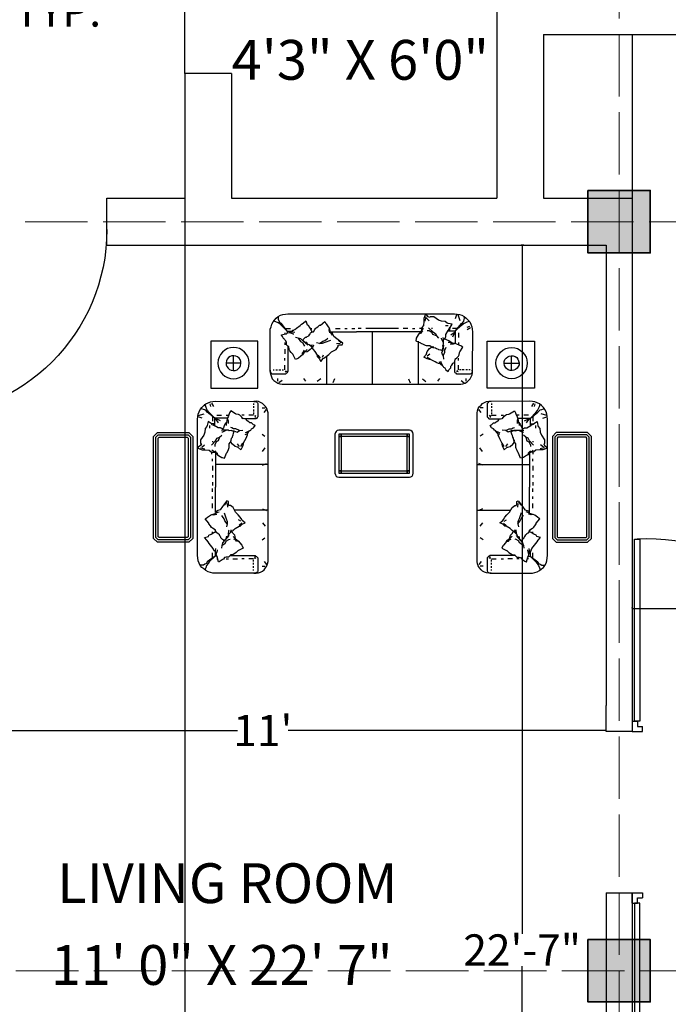
# Model space of a CAD drawing. Units: inches. Extents: x -113 to 5399, y -1393 to 3302.
# Tile 4 of 40: x 1068 to 1193, y 271 to 460. Entities that reach past the tile are written whole.
import ezdxf

# ---------------------------------------------------------------- set-up
doc = ezdxf.new("R2010")
doc.units = ezdxf.units.IN
doc.header["$MEASUREMENT"] = 0
doc.linetypes.add('ACAD_ISO02W100', pattern=[15, 12, -3])
doc.layers.add('24', color=7, linetype='Continuous')
for name, color, linetype, lineweight in [('A-ANNO-DIMS', 254, 'Continuous', 18), ('A-AREA-IDEN', 4, 'Continuous', 18), ('A-COLS', 7, 'Continuous', 35), ('doors', 2, 'Continuous', 25), ('furniture', 131, 'Continuous', 18), ('GRIDS', 7, 'ACAD_ISO02W100', 13), ('walls', 1, 'Continuous', 25)]:
    doc.layers.add(name, color=color, linetype=linetype, lineweight=lineweight)
doc.styles.get("Standard").update_dxf_attribs({"font": 'arial.ttf'})
doc.dimstyles.get("Standard").update_dxf_attribs({"dimtxt": 6, "dimasz": 0.18, "dimexe": 0.18, "dimexo": 0.0625, "dimgap": 0.09, "dimtad": 0, "dimtih": 1, "dimtoh": 1, "dimdec": 1, "dimzin": 0, "dimdsep": 46, "dimlunit": 4, "dimtxsty": 'Standard', "dimblk": 'ARCHTICK', "dimcen": 0.09, "dimadec": 0, "dimazin": 0, "dimtfac": 1, "dimtdec": 1, "dimtofl": 0, "dimtmove": 0, "dimatfit": 3, "dimfxl": 1, "dimtolj": 1, "dimtzin": 0, "dimarcsym": 0})

# ---------------------------------------------------------------- blocks, each defined once
blk = doc.blocks.new('*U3')
for p, q in [((0, 0), (0, -6)), ((36, 0), (36, -6))]:
    blk.add_line(p, q)
blk.add_lwpolyline([(0, 0), (0, 36), (1.75, 36), (1.75, 0)], close=True)
blk.add_arc((0, 0), 36, 0, 90)
blk = doc.blocks.new('DL13712')
at = {"layer": '24'}
for p, q in [((33, 28.5), (-34, 28.5)), ((33.5, -29.5), (-10, -29.5))]:
    blk.add_line(p, q, dxfattribs=at)
blk = doc.blocks.new('DL13976')
at = {"layer": '24'}
for p, q in [((-16, 11), (-13.5, 14)), ((-13.5, 14), (-10.5, 16.5)), ((-10.5, 16.5), (-7, 18.5)), ((-7, 18.5), (-3.5, 19.5)), ((-3.5, 19.5), (0.5, 20)), ((0.5, 20), (4.5, 19.5)), ((4.5, 19.5), (8, 18.5)), ((8, 18.5), (11.5, 16.5)), ((11.5, 16.5), (14.5, 14)), ((14.5, 14), (17, 11)), ((-19.5, 0), (-19, 4)), ((-19, -4), (-19.5, 0)), ((-19, 4), (-18, 7.5)), ((-18, 7.5), (-16, 11)), ((-9, 2), (-8, 4.5)), ((-9, -0.5), (-9, 2)), ((-9, 0), (10, 0)), ((-8, 4.5), (-6.5, 6.5)), ((-6.5, 6.5), (-4.5, 8)), ((-5.5, 0), (6.5, 0)), ((-4.5, 8), (-2.5, 9)), ((-2.5, 9), (0, 9.5)), ((0, 9.5), (2.5, 9.5)), ((0.5, -9.5), (0.5, 9.5)), ((0.5, -6), (0.5, 6)), ((2.5, 9.5), (5, 8.5)), ((5, 8.5), (7, 7)), ((7, 7), (8.5, 5)), ((8.5, 5), (9.5, 3)), ((9.5, 3), (10, 0.5)), ((10, 0.5), (10, -2)), ((17, 11), (19, 7.5)), ((19, 7.5), (20, 4)), ((20, 4), (20.5, 0)), ((20.5, 0), (20, -4)), ((-18, -7.5), (-19, -4)), ((-16, -11), (-18, -7.5)), ((-13.5, -14), (-16, -11)), ((-8.5, -3), (-9, -0.5)), ((-7.5, -5), (-8.5, -3)), ((-6, -7), (-7.5, -5)), ((-4, -8.5), (-6, -7)), ((-1.5, -9.5), (-4, -8.5)), ((1, -9.5), (-1.5, -9.5)), ((3.5, -9), (1, -9.5)), ((5.5, -8), (3.5, -9)), ((7.5, -6.5), (5.5, -8)), ((9, -4.5), (7.5, -6.5)), ((10, -2), (9, -4.5)), ((17, -11), (14.5, -14)), ((19, -7.5), (17, -11)), ((20, -4), (19, -7.5)), ((-10.5, -16.5), (-13.5, -14)), ((-7, -18.5), (-10.5, -16.5)), ((-3.5, -19.5), (-7, -18.5)), ((0.5, -20), (-3.5, -19.5)), ((4.5, -19.5), (0.5, -20)), ((8, -18.5), (4.5, -19.5)), ((11.5, -16.5), (8, -18.5)), ((14.5, -14), (11.5, -16.5))]:
    blk.add_line(p, q, dxfattribs=at)
blk = doc.blocks.new('DL13329')
at = {"layer": '24'}
for p, q in [((0, 0), (0, -60)), ((60, 0), (0, 0)), ((60, -60), (60, 0)), ((0, -60), (60, -60))]:
    blk.add_line(p, q, dxfattribs=at)
blk = doc.blocks.new('DL13303')
at = {"layer": '24'}
for p, q in [((-70, 20), (-65, 25)), ((-70, -20), (-70, 20)), ((-67, 19), (-64, 22)), ((-67, -19), (-67, 19)), ((-65, 25), (65, 25)), ((-64, 22), (64, 22)), ((-64, 18), (-63, 19)), ((-64, -18), (-64, 18)), ((-63, 19), (63, 19)), ((63, 19), (64, 18)), ((64, 22), (67, 19)), ((64, 18), (64, -18)), ((65, 25), (70, 20)), ((67, 19), (67, -19)), ((70, 20), (70, -20)), ((-65, -25), (-70, -20)), ((-64, -22), (-67, -19)), ((65, -25), (-65, -25)), ((-63, -19), (-64, -18)), ((64, -22), (-64, -22)), ((63, -19), (-63, -19)), ((64, -18), (63, -19)), ((67, -19), (64, -22)), ((70, -20), (65, -25))]:
    blk.add_line(p, q, dxfattribs=at)
blk = doc.blocks.new('DL12701')
at = {"layer": '24'}
for p, q in [((-104, 37.5), (-102, 40)), ((-102, 40), (-99.5, 42)), ((-99.5, 42), (-96.5, 43.5)), ((-99, 40), (-99, 42)), ((-99, 38), (-99, 40)), ((-98, 36), (-99, 38)), ((-96.5, 43.5), (-93.5, 44.5)), ((-93.5, 44.5), (-90, 45)), ((-90, 45), (-87, 45.5)), ((-87, 45.5), (0, 45.5)), ((0, 45.5), (87, 45.5)), ((50, 45), (48, 39.5)), ((48, 39.5), (48, 35.5)), ((50.5, 41.5), (49, 36)), ((51.5, 44.5), (50, 45)), ((53.5, 41.5), (51.5, 44.5)), ((51.5, 40), (54.5, 36.5)), ((55.5, 40.5), (53.5, 41.5)), ((56, 41.5), (55.5, 40.5)), ((60.5, 41.5), (56, 41.5)), ((66.5, 37.5), (60.5, 41.5)), ((87, 45.5), (90.5, 45)), ((88.5, 39.5), (90, 44.5)), ((90.5, 45), (93.5, 44.5)), ((91.5, 44.5), (94, 37)), ((93.5, 44.5), (96.5, 43.5)), ((96.5, 43.5), (99.5, 42)), ((99, 36), (99.5, 38)), ((99.5, 42), (102, 40)), ((100, 40), (99.5, 42)), ((99.5, 38), (100, 40)), ((102, 40), (104.5, 37.5)), ((-109.5, 26), (-108.5, 29)), ((-109.5, 22.5), (-109.5, 26)), ((-108.5, 29), (-107.5, 32)), ((-107.5, 32), (-106, 35)), ((-106, 35), (-104, 37.5)), ((-102.5, 35), (-105, 36)), ((-99.5, 34), (-102.5, 35)), ((-97, 32), (-99.5, 34)), ((-97, 34), (-98, 36)), ((-95, 33), (-97, 34)), ((-95, 30.5), (-97, 32)), ((-87.5, 23), (-95, 33)), ((-87.5, 23), (-95, 30.5)), ((-89.5, 26.5), (-83.5, 26.5)), ((-80.5, 24.5), (-78, 25.5)), ((-78, 25.5), (-76, 27)), ((-77, 25.5), (-77, 25.5)), ((-76, 27), (-71.5, 30.5)), ((-71.5, 30.5), (-69.5, 32)), ((-69.5, 32), (-67.5, 33.5)), ((-67.5, 33.5), (-64, 36.5)), ((-64, 36.5), (-62.5, 31.5)), ((-62.5, 31.5), (-61, 31)), ((-61, 31), (-59.5, 28)), ((-59.5, 28), (-57.5, 24.5)), ((-58, 26.5), (-56.5, 26.5)), ((-54.5, 22.5), (-52.5, 25.5)), ((-52.5, 25.5), (-52, 26.5)), ((-52, 26.5), (-51, 27.5)), ((-51, 27.5), (-49, 29)), ((-49, 29), (-46.5, 31)), ((-46.5, 31), (-45.5, 31)), ((-45.5, 31), (-40, 35.5)), ((-40, 35.5), (-38.5, 33)), ((-38.5, 33), (-38, 32.5)), ((-38, 32.5), (-35.5, 29)), ((-35.5, 29), (-34.5, 27)), ((-34.5, 27), (-35, 24.5)), ((-34.5, 27), (-33.5, 24)), ((-26.5, 26.5), (-20.5, 26.5)), ((-14.5, 26.5), (-11.5, 26.5)), ((-5.5, 26.5), (-1.5, 26.5)), ((6.5, 26.5), (2.5, 26.5)), ((15.5, 26.5), (12.5, 26.5)), ((27.5, 26.5), (21.5, 26.5)), ((33.5, 26.5), (36.5, 26.5)), ((42.5, 27), (45, 27)), ((45.5, 28), (45, 27)), ((45, 27), (45, 23.5)), ((45, 23.5), (46.5, 26)), ((47.5, 30.5), (45.5, 28)), ((46.5, 26), (47.5, 27)), ((48, 35.5), (47.5, 30.5)), ((54, 27.5), (59.5, 22.5)), ((59, 26.5), (57.5, 26.5)), ((70.5, 36), (66.5, 37.5)), ((75, 35.5), (70.5, 36)), ((77.5, 33.5), (75, 35.5)), ((79, 30), (75.5, 30)), ((79, 33), (77.5, 33.5)), ((84, 32), (79, 33)), ((80.5, 28), (79, 24)), ((81, 24.5), (81.5, 28)), ((81.5, 28), (84, 32)), ((90.5, 26.5), (84.5, 26.5)), ((88.5, 23.5), (96, 33)), ((88.5, 23.5), (95.5, 30.5)), ((95.5, 30.5), (98, 32.5)), ((96, 33), (97.5, 34.5)), ((97.5, 34.5), (99, 36)), ((98, 32.5), (100.5, 34)), ((100.5, 34), (103, 35)), ((103, 35), (106, 36)), ((103, 28.5), (106.5, 29.5)), ((107.5, 27.5), (103, 25)), ((104.5, 37.5), (106.5, 35)), ((106.5, 35), (108, 32)), ((108, 32), (109, 29)), ((109, 29), (109.5, 26)), ((109.5, 26), (110, 22.5)), ((-109.5, -26.5), (-109.5, 22.5)), ((-95, 18.5), (-92, 19.5)), ((-95, 18), (-95, 18.5)), ((-94, 16.5), (-95, 18)), ((-92.5, 14), (-94, 16.5)), ((-92, 13.5), (-92.5, 14)), ((-92, 19.5), (-89, 20)), ((-91.5, 12.5), (-92, 13.5)), ((-91, 21), (-91, 19.5)), ((-89, 20), (-87.5, 21)), ((-87.5, 21), (-87.5, 23)), ((-81.5, 23), (-87.5, 23)), ((-87.5, 21), (-85, 21.5)), ((-85, 21.5), (-82, 22.5)), ((-85, 21.5), (-80.5, 20)), ((-82, 22.5), (-80.5, 24.5)), ((-82, 22.5), (-80.5, 22.5)), ((-80.5, 24.5), (-80.5, 23.5)), ((-80.5, 22.5), (-78, 22)), ((-80.5, 20), (-79.5, 20)), ((-74, 14.5), (-77.5, 15)), ((-70.5, 13.5), (-74, 14.5)), ((-74, 14.5), (-71, 10)), ((-67.5, 10.5), (-70.5, 13.5)), ((-67.5, 12.5), (-66.5, 13.5)), ((-66.5, 13.5), (-64.5, 15.5)), ((-64.5, 15.5), (-63.5, 15.5)), ((-63.5, 15.5), (-62.5, 16.5)), ((-62.5, 16.5), (-60.5, 17.5)), ((-60.5, 17.5), (-59, 19.5)), ((-59, 19.5), (-58.5, 19.5)), ((-58.5, 19.5), (-58, 21)), ((-58, 21), (-54.5, 23)), ((-57.5, 24.5), (-56.5, 22)), ((-56.5, 22.5), (-54.5, 22.5)), ((-54.5, 23), (-54.5, 22.5)), ((-54, 22.5), (-54, 22.5)), ((-40, 11.5), (-37, 13.5)), ((-37, 13.5), (-36, 14.5)), ((-35, 24.5), (-34.5, 23)), ((-34.5, 23), (-34, 21)), ((-33.5, 24), (-33, 22)), ((-30, 21), (-33, 22)), ((-33, 22), (-31.5, 19.5)), ((-32, 22.5), (0.5, 22.5)), ((-31.5, 19.5), (-31, 18)), ((-29.5, 19.5), (-30, 21)), ((-28.5, 16.5), (-29.5, 19.5)), ((-24.5, 13.5), (-28.5, 16.5)), ((-21, 11), (-24.5, 13.5)), ((44, 22.5), (0.5, 22.5)), ((38, 14), (37.5, 11)), ((40.5, 18.5), (38, 14.5)), ((38, 14.5), (38, 14)), ((41.5, 20), (40.5, 18.5)), ((43.5, 22), (41.5, 20)), ((43.5, 20.5), (41.5, 20)), ((45, 23.5), (43.5, 22)), ((45, 22), (43.5, 20.5)), ((46.5, 23.5), (45, 22)), ((54.5, 23.5), (52, 23.5)), ((58, 21.5), (54.5, 23.5)), ((59.5, 19), (58, 21.5)), ((59.5, 22.5), (63, 20.5)), ((64, 17.5), (59.5, 19)), ((63, 20.5), (64, 17.5)), ((64, 17.5), (66.5, 14.5)), ((70.5, 13.5), (70.5, 14.5)), ((73, 8.5), (70.5, 13.5)), ((73, 13), (72.5, 15)), ((73, 12.5), (75, 14.5)), ((73, 12.5), (73, 13)), ((76, 12.5), (74, 14)), ((75, 14.5), (76, 16)), ((75.5, 16), (76, 16.5)), ((76, 19), (79, 24)), ((76, 16), (76, 19)), ((79, 24), (81, 24.5)), ((79, 23.5), (88.5, 23.5)), ((82.5, 18.5), (88, 22.5)), ((85, 16), (88, 22.5)), ((88.5, 8), (88.5, 23.5)), ((92, 21), (92, 15)), ((110, 22.5), (109.5, -26.5)), ((-89.5, 11), (-91.5, 12.5)), ((-91, 9), (-91, 6)), ((-91, 0.5), (-91, -5.5)), ((-89, 9), (-89.5, 11)), ((-89, 8.5), (-89, 9)), ((-89, 6), (-89, 8.5)), ((-86.5, 3.5), (-89, 6)), ((-87, 3.5), (-87, -26.5)), ((-86, 3.5), (-86.5, 3.5)), ((-85.5, 0.5), (-86, 3.5)), ((-85.5, 0), (-85.5, 0.5)), ((-84.5, -2), (-85.5, 0)), ((-71, 10), (-68, 8.5)), ((-68, 12), (-67.5, 12.5)), ((-65, 9), (-68, 12)), ((-68, 8.5), (-66.5, 5.5)), ((-61.5, 5.5), (-67.5, 10.5)), ((-66.5, 5.5), (-66, 4)), ((-63, 9), (-65, 9)), ((-62.5, 0), (-63.5, -1)), ((-62, 6.5), (-63, 9)), ((-60, 6), (-62, 6.5)), ((-61, -2), (-58.5, 0.5)), ((-57.5, 3.5), (-60, 6)), ((-60, 6), (-55, 5.5)), ((-58.5, 0.5), (-55.5, 2)), ((-56.5, 3.5), (-57.5, 3.5)), ((-57.5, 3.5), (-56, 1.5)), ((-54, 3), (-56.5, 3.5)), ((-56, 1.5), (-55, 0)), ((-55, 5.5), (-54, 5)), ((-55, 0), (-52.5, -2.5)), ((-46.5, 7.5), (-50.5, 8.5)), ((-46.5, 7.5), (-42.5, 10.5)), ((-43.5, 7.5), (-46.5, 7.5)), ((-40, 9), (-43.5, 7.5)), ((-42.5, 10.5), (-40, 11.5)), ((-32.5, 11.5), (-40, 9)), ((-31.5, -3), (-25.5, 0)), ((-25.5, 0), (-23, 3.5)), ((-20.5, 7.5), (-25, 7)), ((-23, 5.5), (-21.5, 6)), ((-23, 3.5), (-23, 5.5)), ((-19, 8.5), (-22.5, 11.5)), ((-21.5, 6), (-18, 6)), ((-17, 8), (-21, 11)), ((-18, 6), (-17, 8)), ((37.5, 11), (43.5, 8.5)), ((43.5, 8.5), (44, 8)), ((44, 8), (47, 6.5)), ((47, 6.5), (49.5, 5.5)), ((49.5, 5.5), (51, 5)), ((51, 5), (52.5, 5)), ((52, -2.5), (55, 1)), ((52.5, 5), (55.5, 5)), ((55, 1), (57.5, 3)), ((55.5, 5), (55.5, 5)), ((55.5, 5), (59, 2.5)), ((59, 2.5), (60, 3.5)), ((60, 3.5), (60, 2.5)), ((60, 2.5), (63, 2)), ((63, 2), (64, 1)), ((64, 1), (66, 0.5)), ((66, 0.5), (66.5, 0)), ((66.5, 0), (69, -0.5)), ((71.5, -1), (72.5, 2.5)), ((72, 5), (73, 6.5)), ((73, 5.5), (72, -1)), ((72.5, 2.5), (72, 5)), ((73, 8.5), (73, 12.5)), ((73, 6.5), (73, 8.5)), ((74.5, -0.5), (76, 1.5)), ((80, 11), (76, 12.5)), ((76, 1.5), (76.5, 3)), ((80.5, 9), (79, 9)), ((80.5, 10.5), (80, 11)), ((83, 8.5), (80.5, 10.5)), ((83, 8.5), (80.5, 9)), ((84, 6.5), (81.5, 6.5)), ((85, 8), (83, 8.5)), ((85.5, 6.5), (84, 6.5)), ((88, 7.5), (85, 8)), ((88, 7.5), (85.5, 6.5)), ((90, 6.5), (88, 7.5)), ((94, 5), (90, 6.5)), ((92, 9), (92, 6)), ((95, 4.5), (94, 5)), ((94, -3), (97.5, 3)), ((97.5, 3), (95, 4.5)), ((-91, -14), (-91, -11)), ((-83, -4), (-84.5, -2)), ((-80.5, -6.5), (-83, -4)), ((-80.5, -7), (-80.5, -6.5)), ((-77.5, -13), (-80.5, -7)), ((-74.5, -11.5), (-77.5, -13)), ((-73.5, -11), (-74.5, -11.5)), ((-70.5, -8.5), (-73.5, -11)), ((-68.5, -7), (-70.5, -8.5)), ((-68.5, -4.5), (-67, -3)), ((-66.5, -4.5), (-68.5, -7)), ((-68.5, -7), (-68.5, -4.5)), ((-67, -3), (-66, -1)), ((-65.5, -3), (-66.5, -4.5)), ((-63.5, -1), (-65.5, -3)), ((-65.5, -3), (-62.5, -2.5)), ((-62.5, -2.5), (-61, -2)), ((-54, -0.5), (-53.5, -0.5)), ((-52.5, -2.5), (-49.5, -7.5)), ((-49.5, -7.5), (-49.5, -9)), ((-49.5, -9), (-47, -11.5)), ((-45.5, -11), (-48.5, -7.5)), ((-47, -11.5), (-45, -15.5)), ((-45, -15.5), (-42, -11.5)), ((-43, -10), (-41.5, -7)), ((-42, -11.5), (-41, -11)), ((-41, -11), (-38, -9)), ((-38, -9), (-35, -6.5)), ((-35, -6.5), (-31.5, -3)), ((48, -10), (51.5, -6)), ((52, -12), (48, -10)), ((51.5, -5.5), (52, -2.5)), ((51.5, -6), (51.5, -5.5)), ((52, -8), (55.5, -5.5)), ((52, -10), (56.5, -12.5)), ((55, -13), (52, -12)), ((69, -0.5), (70.5, -1)), ((70.5, -1), (71.5, -1)), ((72, -1), (70.5, -5)), ((70.5, -5), (72.5, -8)), ((72.5, -8), (74.5, -3.5)), ((72.5, -8), (73, -12.5)), ((74.5, -3.5), (74.5, -0.5)), ((87.5, -12.5), (89.5, -11)), ((88, -13), (87.5, -12.5)), ((89.5, -11), (91, -10)), ((91, -10), (92, -8.5)), ((92, -8.5), (93, -7)), ((92, -14), (92, -11)), ((93, -7), (93.5, -4)), ((93.5, -4), (94, -3)), ((-91, -26), (-91, -20)), ((56.5, -13), (55, -13)), ((62.5, -16), (56.5, -13)), ((64.5, -17), (62.5, -16)), ((64, -16.5), (64, -16.5)), ((66.5, -18), (64.5, -17)), ((69, -18.5), (66.5, -18)), ((67.5, -15.5), (68.5, -18)), ((68.5, -18), (69, -18.5)), ((69, -18.5), (72, -21)), ((70, -16.5), (69.5, -15.5)), ((72, -21), (70, -16.5)), ((72, -21), (73, -22.5)), ((73, -22.5), (74.5, -23.5)), ((74.5, -23.5), (76, -26)), ((80, -26), (82.5, -23.5)), ((82.5, -21.5), (83.5, -20)), ((82.5, -22.5), (82.5, -21.5)), ((82.5, -23.5), (82.5, -22.5)), ((83.5, -20), (85, -18)), ((85, -17.5), (87, -16.5)), ((85, -18), (85, -17.5)), ((87, -16.5), (88, -13)), ((87.5, -26.5), (87.5, -14.5)), ((92, -26), (92, -20)), ((-109.5, -28), (-109.5, -26.5)), ((-109.5, -26.5), (-109.5, -29.5)), ((-109, -29), (-109.5, -28)), ((-109.5, -29.5), (-109, -32.5)), ((-108.5, -30), (-109, -29)), ((-109, -32.5), (-108, -35)), ((-108, -31), (-108.5, -30)), ((-106.5, -31.5), (-108, -31)), ((-108, -35), (-107, -37.5)), ((-107, -37.5), (-105, -39.5)), ((-105.5, -31.5), (-106.5, -31.5)), ((-106, -26), (-104.5, -26)), ((-104.5, -31.5), (-105.5, -31.5)), ((-92, -31.5), (-104.5, -31.5)), ((-102.5, -26), (-100.5, -26)), ((-100.5, -37), (-100.5, -40.5)), ((-98.5, -26), (-96, -26)), ((-94.5, -26), (-92.5, -26)), ((-91, -31.5), (-92, -31.5)), ((-90, -31.5), (-91, -31.5)), ((-90.5, -27.5), (-88, -28)), ((-90.5, -28), (-90, -29)), ((-89, -30.5), (-90, -31.5)), ((-88, -30), (-89, -30.5)), ((-87.5, -29), (-88, -30)), ((-87, -28), (-87.5, -29)), ((-87, -26.5), (-87, -28)), ((-67, -37), (-64.5, -40.5)), ((-45, -37.5), (-49.5, -41)), ((-27.5, -37.5), (-29.5, -42.5)), ((28.5, -37.5), (30.5, -42.5)), ((46, -37.5), (50.5, -41)), ((68, -37), (65.5, -40.5)), ((76, -26), (79, -28)), ((79, -28), (79.5, -27.5)), ((79.5, -27.5), (80, -26)), ((87.5, -28), (87.5, -26.5)), ((87.5, -29), (87.5, -28)), ((88, -30), (87.5, -29)), ((89, -30.5), (88, -30)), ((91.5, -27.5), (89, -28)), ((90, -31.5), (89, -30.5)), ((91, -31.5), (90, -31.5)), ((91.5, -28), (91, -29)), ((92.5, -31.5), (91, -31.5)), ((104.5, -31.5), (92.5, -31.5)), ((95.5, -26), (93.5, -26)), ((99.5, -26), (97, -26)), ((103.5, -26), (101.5, -26)), ((101.5, -37), (101.5, -40.5)), ((106, -31.5), (104.5, -31.5)), ((105, -39.5), (107, -37.5)), ((107, -26), (105.5, -26)), ((107, -31.5), (106, -31.5)), ((108, -31), (107, -31.5)), ((107, -37.5), (108.5, -35)), ((109, -30), (108, -31)), ((108.5, -35), (109.5, -32.5)), ((109.5, -29), (109, -30)), ((110, -29.5), (109.5, -26.5)), ((109.5, -26.5), (109.5, -28)), ((109.5, -28), (109.5, -29)), ((109.5, -32.5), (110, -29.5)), ((-105, -39.5), (-102.5, -41.5)), ((-102.5, -41.5), (-100, -43)), ((-100, -43), (-97.5, -44)), ((-94.5, -39.5), (-98.5, -42.5)), ((-97.5, -44), (-94.5, -44.5)), ((-94.5, -44.5), (0, -44.5)), ((0, -44.5), (95, -44.5)), ((95, -44.5), (97.5, -44)), ((95.5, -39.5), (99.5, -42.5)), ((97.5, -44), (100.5, -43)), ((100.5, -43), (103, -41.5)), ((103, -41.5), (105, -39.5))]:
    blk.add_line(p, q, dxfattribs=at)
blk = doc.blocks.new('DL13707')
at = {"layer": '24'}
for p, q in [((0, -33.5), (0, 33.5)), ((-58.5, -33.5), (-58.5, 21.5)), ((58.5, -33.5), (58.5, 2))]:
    blk.add_line(p, q, dxfattribs=at)
blk = doc.blocks.new('DL13651')
at = {"layer": '24'}
for p, q in [((-50.5, 25), (-50, 27)), ((-50, 27), (-49, 28.5)), ((-49, 28.5), (-47.5, 29.5)), ((-47.5, 29.5), (-45.5, 30)), ((-45.5, 30), (44.5, 30)), ((44.5, 30), (46.5, 29.5)), ((46.5, 29.5), (48, 28.5)), ((48, 28.5), (49, 27)), ((49, 27), (49.5, 25)), ((-50.5, -25), (-50.5, 25)), ((-45.5, 24.5), (-45.5, 25)), ((-45.5, 25), (-45, 25)), ((-45.5, -24.5), (-45.5, 24.5)), ((-45, 25), (44, 25)), ((-45, 22), (44, 22)), ((-42.5, 22), (-45, 22)), ((-42.5, -24.5), (-42.5, 24.5)), ((-42.5, 24.5), (-42.5, 22)), ((41.5, 22), (41.5, 24.5)), ((41.5, 24.5), (41.5, -24.5)), ((44, 22), (41.5, 22)), ((44, 25), (44.5, 25)), ((44.5, 25), (44.5, 24.5)), ((44.5, 24.5), (44.5, -24.5)), ((49.5, 25), (49.5, -25)), ((-50, -27), (-50.5, -25)), ((-45.5, -25), (-45.5, -24.5)), ((-45, -25), (-45.5, -25)), ((44, -22), (-45, -22)), ((-45, -22), (-42.5, -22)), ((44, -25), (-45, -25)), ((-42.5, -22), (-42.5, -24.5)), ((41.5, -24.5), (41.5, -22)), ((41.5, -22), (44, -22)), ((44.5, -25), (44, -25)), ((44.5, -24.5), (44.5, -25)), ((49.5, -25), (49, -27)), ((-49, -28.5), (-50, -27)), ((-47.5, -29.5), (-49, -28.5)), ((-45.5, -30), (-47.5, -29.5)), ((44.5, -30), (-45.5, -30)), ((46.5, -29.5), (44.5, -30)), ((48, -28.5), (46.5, -29.5)), ((49, -27), (48, -28.5))]:
    blk.add_line(p, q, dxfattribs=at)
blk = doc.blocks.new('DL12263')
at = {"layer": '24'}
for p, q in [((-123, 37.5), (-121, 40)), ((-121, 40), (-118.5, 42)), ((-118.5, 42), (-115.5, 43.5)), ((-118, 40), (-118, 42)), ((-118, 38), (-118, 40)), ((-117, 36), (-118, 38)), ((-115.5, 43.5), (-112.5, 44.5)), ((-112.5, 44.5), (-109, 45)), ((-109, 45), (-106, 45.5)), ((-106, 45.5), (-19, 45.5)), ((-19, 45.5), (106.5, 45.5)), ((69.5, 45), (67.5, 39.5)), ((67.5, 39.5), (67.5, 35.5)), ((70, 41.5), (68.5, 36)), ((71, 44.5), (69.5, 45)), ((73, 41.5), (71, 44.5)), ((71, 40), (74, 36.5)), ((75, 40.5), (73, 41.5)), ((75.5, 41.5), (75, 40.5)), ((80, 41.5), (75.5, 41.5)), ((86, 37.5), (80, 41.5)), ((106.5, 45.5), (110, 45)), ((108, 39.5), (109.5, 44.5)), ((110, 45), (113, 44.5)), ((111, 44.5), (113.5, 37)), ((113, 44.5), (116, 43.5)), ((116, 43.5), (119, 42)), ((118.5, 36), (119, 38)), ((119, 42), (121.5, 40)), ((119.5, 40), (119, 42)), ((119, 38), (119.5, 40)), ((121.5, 40), (124, 37.5)), ((-128.5, 26), (-127.5, 29)), ((-128.5, 22.5), (-128.5, 26)), ((-127.5, 29), (-126.5, 32)), ((-126.5, 32), (-125, 35)), ((-125, 35), (-123, 37.5)), ((-121.5, 35), (-124, 36)), ((-118.5, 34), (-121.5, 35)), ((-116, 32), (-118.5, 34)), ((-116, 34), (-117, 36)), ((-114, 33), (-116, 34)), ((-114, 30.5), (-116, 32)), ((-106.5, 23), (-114, 33)), ((-106.5, 23), (-114, 30.5)), ((-108.5, 26.5), (-102.5, 26.5)), ((-99.5, 24.5), (-97, 25.5)), ((-97, 25.5), (-95, 27)), ((-96, 25.5), (-96, 25.5)), ((-95, 27), (-90.5, 30.5)), ((-90.5, 30.5), (-88.5, 32)), ((-88.5, 32), (-86.5, 33.5)), ((-86.5, 33.5), (-83, 36.5)), ((-83, 36.5), (-81.5, 31.5)), ((-81.5, 31.5), (-80, 31)), ((-80, 31), (-78.5, 28)), ((-78.5, 28), (-76.5, 24.5)), ((-77, 26.5), (-75.5, 26.5)), ((-73.5, 22.5), (-71.5, 25.5)), ((-71.5, 25.5), (-71, 26.5)), ((-71, 26.5), (-70, 27.5)), ((-70, 27.5), (-68, 29)), ((-68, 29), (-65.5, 31)), ((-65.5, 31), (-64.5, 31)), ((-64.5, 31), (-59, 35.5)), ((-59, 35.5), (-57.5, 33)), ((-57.5, 33), (-57, 32.5)), ((-57, 32.5), (-54.5, 29)), ((-54.5, 29), (-53.5, 27)), ((-53.5, 27), (-54, 24.5)), ((-53.5, 27), (-52.5, 24)), ((-45.5, 26.5), (-39.5, 26.5)), ((-33.5, 26.5), (-30.5, 26.5)), ((-24.5, 26.5), (-20.5, 26.5)), ((-12.5, 26.5), (-16.5, 26.5)), ((35, 26.5), (-6.5, 26.5)), ((47, 26.5), (41, 26.5)), ((53, 26.5), (56, 26.5)), ((62, 27), (64.5, 27)), ((65, 28), (64.5, 27)), ((64.5, 27), (64.5, 23.5)), ((64.5, 23.5), (66, 26)), ((67, 30.5), (65, 28)), ((66, 26), (67, 27)), ((67.5, 35.5), (67, 30.5)), ((73.5, 27.5), (79, 22.5)), ((78.5, 26.5), (77, 26.5)), ((90, 36), (86, 37.5)), ((94.5, 35.5), (90, 36)), ((97, 33.5), (94.5, 35.5)), ((98.5, 30), (95, 30)), ((98.5, 33), (97, 33.5)), ((103.5, 32), (98.5, 33)), ((100, 28), (98.5, 24)), ((100.5, 24.5), (101, 28)), ((101, 28), (103.5, 32)), ((110, 26.5), (104, 26.5)), ((108, 23.5), (115.5, 33)), ((108, 23.5), (115, 30.5)), ((115, 30.5), (117.5, 32.5)), ((115.5, 33), (117, 34.5)), ((117, 34.5), (118.5, 36)), ((117.5, 32.5), (120, 34)), ((120, 34), (122.5, 35)), ((122.5, 35), (125.5, 36)), ((122.5, 28.5), (126, 29.5)), ((127, 27.5), (122.5, 25)), ((124, 37.5), (126, 35)), ((126, 35), (127.5, 32)), ((127.5, 32), (128.5, 29)), ((128.5, 29), (129, 26)), ((129, 26), (129.5, 22.5)), ((-128.5, -26.5), (-128.5, 22.5)), ((-114, 18.5), (-111, 19.5)), ((-114, 18), (-114, 18.5)), ((-113, 16.5), (-114, 18)), ((-111.5, 14), (-113, 16.5)), ((-111, 13.5), (-111.5, 14)), ((-111, 19.5), (-108, 20)), ((-110.5, 12.5), (-111, 13.5)), ((-110, 21), (-110, 19.5)), ((-108, 20), (-106.5, 21)), ((-106.5, 21), (-106.5, 23)), ((-100.5, 23), (-106.5, 23)), ((-106.5, 21), (-104, 21.5)), ((-104, 21.5), (-101, 22.5)), ((-104, 21.5), (-99.5, 20)), ((-101, 22.5), (-99.5, 24.5)), ((-101, 22.5), (-99.5, 22.5)), ((-99.5, 24.5), (-99.5, 23.5)), ((-99.5, 22.5), (-97, 22)), ((-99.5, 20), (-98.5, 20)), ((-93, 14.5), (-96.5, 15)), ((-89.5, 13.5), (-93, 14.5)), ((-93, 14.5), (-90, 10)), ((-86.5, 10.5), (-89.5, 13.5)), ((-86.5, 12.5), (-85.5, 13.5)), ((-85.5, 13.5), (-83.5, 15.5)), ((-83.5, 15.5), (-82.5, 15.5)), ((-82.5, 15.5), (-81.5, 16.5)), ((-81.5, 16.5), (-79.5, 17.5)), ((-79.5, 17.5), (-78, 19.5)), ((-78, 19.5), (-77.5, 19.5)), ((-77.5, 19.5), (-77, 21)), ((-77, 21), (-73.5, 23)), ((-76.5, 24.5), (-75.5, 22)), ((-75.5, 22.5), (-73.5, 22.5)), ((-73.5, 23), (-73.5, 22.5)), ((-73, 22.5), (-73, 22.5)), ((-59, 11.5), (-56, 13.5)), ((-56, 13.5), (-55, 14.5)), ((-54, 24.5), (-53.5, 23)), ((-53.5, 23), (-53, 21)), ((-52.5, 24), (-52, 22)), ((-49, 21), (-52, 22)), ((-52, 22), (-50.5, 19.5)), ((-51, 22.5), (-18.5, 22.5)), ((-50.5, 19.5), (-50, 18)), ((-48.5, 19.5), (-49, 21)), ((-47.5, 16.5), (-48.5, 19.5)), ((-43.5, 13.5), (-47.5, 16.5)), ((-40, 11), (-43.5, 13.5)), ((63.5, 22.5), (-18.5, 22.5)), ((57.5, 14), (57, 11)), ((60, 18.5), (57.5, 14.5)), ((57.5, 14.5), (57.5, 14)), ((61, 20), (60, 18.5)), ((63, 22), (61, 20)), ((63, 20.5), (61, 20)), ((64.5, 23.5), (63, 22)), ((64.5, 22), (63, 20.5)), ((66, 23.5), (64.5, 22)), ((74, 23.5), (71.5, 23.5)), ((77.5, 21.5), (74, 23.5)), ((79, 19), (77.5, 21.5)), ((79, 22.5), (82.5, 20.5)), ((83.5, 17.5), (79, 19)), ((82.5, 20.5), (83.5, 17.5)), ((83.5, 17.5), (86, 14.5)), ((90, 13.5), (90, 14.5)), ((92.5, 8.5), (90, 13.5)), ((92.5, 13), (92, 15)), ((92.5, 12.5), (94.5, 14.5)), ((92.5, 12.5), (92.5, 13)), ((95.5, 12.5), (93.5, 14)), ((94.5, 14.5), (95.5, 16)), ((95, 16), (95.5, 16.5)), ((95.5, 19), (98.5, 24)), ((95.5, 16), (95.5, 19)), ((98.5, 24), (100.5, 24.5)), ((98.5, 23.5), (108, 23.5)), ((102, 18.5), (107.5, 22.5)), ((104.5, 16), (107.5, 22.5)), ((108, 8), (108, 23.5)), ((111.5, 21), (111.5, 15)), ((129.5, 22.5), (129, -26.5)), ((-108.5, 11), (-110.5, 12.5)), ((-110, 9), (-110, 6)), ((-110, 0.5), (-110, -5.5)), ((-108, 9), (-108.5, 11)), ((-108, 8.5), (-108, 9)), ((-108, 6), (-108, 8.5)), ((-105.5, 3.5), (-108, 6)), ((-106, 3.5), (-106, -26.5)), ((-105, 3.5), (-105.5, 3.5)), ((-104.5, 0.5), (-105, 3.5)), ((-104.5, 0), (-104.5, 0.5)), ((-103.5, -2), (-104.5, 0)), ((-90, 10), (-87, 8.5)), ((-87, 12), (-86.5, 12.5)), ((-84, 9), (-87, 12)), ((-87, 8.5), (-85.5, 5.5)), ((-80.5, 5.5), (-86.5, 10.5)), ((-85.5, 5.5), (-85, 4)), ((-82, 9), (-84, 9)), ((-81.5, 0), (-82.5, -1)), ((-81, 6.5), (-82, 9)), ((-79, 6), (-81, 6.5)), ((-80, -2), (-77.5, 0.5)), ((-76.5, 3.5), (-79, 6)), ((-79, 6), (-74, 5.5)), ((-77.5, 0.5), (-74.5, 2)), ((-75.5, 3.5), (-76.5, 3.5)), ((-76.5, 3.5), (-75, 1.5)), ((-73, 3), (-75.5, 3.5)), ((-75, 1.5), (-74, 0)), ((-74, 5.5), (-73, 5)), ((-74, 0), (-71.5, -2.5)), ((-65.5, 7.5), (-69.5, 8.5)), ((-65.5, 7.5), (-61.5, 10.5)), ((-62.5, 7.5), (-65.5, 7.5)), ((-59, 9), (-62.5, 7.5)), ((-61.5, 10.5), (-59, 11.5)), ((-51.5, 11.5), (-59, 9)), ((-50.5, -3), (-44.5, 0)), ((-44.5, 0), (-42, 3.5)), ((-39.5, 7.5), (-44, 7)), ((-42, 5.5), (-40.5, 6)), ((-42, 3.5), (-42, 5.5)), ((-38, 8.5), (-41.5, 11.5)), ((-40.5, 6), (-37, 6)), ((-36, 8), (-40, 11)), ((-37, 6), (-36, 8)), ((57, 11), (63, 8.5)), ((63, 8.5), (63.5, 8)), ((63.5, 8), (66.5, 6.5)), ((66.5, 6.5), (69, 5.5)), ((69, 5.5), (70.5, 5)), ((70.5, 5), (72, 5)), ((71.5, -2.5), (74.5, 1)), ((72, 5), (75, 5)), ((74.5, 1), (77, 3)), ((75, 5), (75, 5)), ((75, 5), (78.5, 2.5)), ((78.5, 2.5), (79.5, 3.5)), ((79.5, 3.5), (79.5, 2.5)), ((79.5, 2.5), (82.5, 2)), ((82.5, 2), (83.5, 1)), ((83.5, 1), (85.5, 0.5)), ((85.5, 0.5), (86, 0)), ((86, 0), (88.5, -0.5)), ((91, -1), (92, 2.5)), ((91.5, 5), (92.5, 6.5)), ((92.5, 5.5), (91.5, -1)), ((92, 2.5), (91.5, 5)), ((92.5, 8.5), (92.5, 12.5)), ((92.5, 6.5), (92.5, 8.5)), ((94, -0.5), (95.5, 1.5)), ((99.5, 11), (95.5, 12.5)), ((95.5, 1.5), (96, 3)), ((100, 9), (98.5, 9)), ((100, 10.5), (99.5, 11)), ((102.5, 8.5), (100, 10.5)), ((102.5, 8.5), (100, 9)), ((103.5, 6.5), (101, 6.5)), ((104.5, 8), (102.5, 8.5)), ((105, 6.5), (103.5, 6.5)), ((107.5, 7.5), (104.5, 8)), ((107.5, 7.5), (105, 6.5)), ((109.5, 6.5), (107.5, 7.5)), ((113.5, 5), (109.5, 6.5)), ((111.5, 9), (111.5, 6)), ((114.5, 4.5), (113.5, 5)), ((113.5, -3), (117, 3)), ((117, 3), (114.5, 4.5)), ((-110, -14), (-110, -11)), ((-102, -4), (-103.5, -2)), ((-99.5, -6.5), (-102, -4)), ((-99.5, -7), (-99.5, -6.5)), ((-96.5, -13), (-99.5, -7)), ((-93.5, -11.5), (-96.5, -13)), ((-92.5, -11), (-93.5, -11.5)), ((-89.5, -8.5), (-92.5, -11)), ((-87.5, -7), (-89.5, -8.5)), ((-87.5, -4.5), (-86, -3)), ((-85.5, -4.5), (-87.5, -7)), ((-87.5, -7), (-87.5, -4.5)), ((-86, -3), (-85, -1)), ((-84.5, -3), (-85.5, -4.5)), ((-82.5, -1), (-84.5, -3)), ((-84.5, -3), (-81.5, -2.5)), ((-81.5, -2.5), (-80, -2)), ((-73, -0.5), (-72.5, -0.5)), ((-71.5, -2.5), (-68.5, -7.5)), ((-68.5, -7.5), (-68.5, -9)), ((-68.5, -9), (-66, -11.5)), ((-64.5, -11), (-67.5, -7.5)), ((-66, -11.5), (-64, -15.5)), ((-64, -15.5), (-61, -11.5)), ((-62, -10), (-60.5, -7)), ((-61, -11.5), (-60, -11)), ((-60, -11), (-57, -9)), ((-57, -9), (-54, -6.5)), ((-54, -6.5), (-50.5, -3)), ((67.5, -10), (71, -6)), ((71.5, -12), (67.5, -10)), ((71, -5.5), (71.5, -2.5)), ((71, -6), (71, -5.5)), ((71.5, -8), (75, -5.5)), ((71.5, -10), (76, -12.5)), ((74.5, -13), (71.5, -12)), ((88.5, -0.5), (90, -1)), ((90, -1), (91, -1)), ((91.5, -1), (90, -5)), ((90, -5), (92, -8)), ((92, -8), (94, -3.5)), ((92, -8), (92.5, -12.5)), ((94, -3.5), (94, -0.5)), ((107, -12.5), (109, -11)), ((107.5, -13), (107, -12.5)), ((109, -11), (110.5, -10)), ((110.5, -10), (111.5, -8.5)), ((111.5, -8.5), (112.5, -7)), ((111.5, -14), (111.5, -11)), ((112.5, -7), (113, -4)), ((113, -4), (113.5, -3)), ((-110, -26), (-110, -20)), ((76, -13), (74.5, -13)), ((82, -16), (76, -13)), ((84, -17), (82, -16)), ((83.5, -16.5), (83.5, -16.5)), ((86, -18), (84, -17)), ((88.5, -18.5), (86, -18)), ((87, -15.5), (88, -18)), ((88, -18), (88.5, -18.5)), ((88.5, -18.5), (91.5, -21)), ((89.5, -16.5), (89, -15.5)), ((91.5, -21), (89.5, -16.5)), ((91.5, -21), (92.5, -22.5)), ((92.5, -22.5), (94, -23.5)), ((94, -23.5), (95.5, -26)), ((99.5, -26), (102, -23.5)), ((102, -21.5), (103, -20)), ((102, -22.5), (102, -21.5)), ((102, -23.5), (102, -22.5)), ((103, -20), (104.5, -18)), ((104.5, -17.5), (106.5, -16.5)), ((104.5, -18), (104.5, -17.5)), ((106.5, -16.5), (107.5, -13)), ((107, -26.5), (107, -14.5)), ((111.5, -26), (111.5, -20)), ((-128.5, -28), (-128.5, -26.5)), ((-128.5, -26.5), (-128.5, -29.5)), ((-128, -29), (-128.5, -28)), ((-128.5, -29.5), (-128, -32.5)), ((-127.5, -30), (-128, -29)), ((-128, -32.5), (-127, -35)), ((-127, -31), (-127.5, -30)), ((-125.5, -31.5), (-127, -31)), ((-127, -35), (-126, -37.5)), ((-126, -37.5), (-124, -39.5)), ((-124.5, -31.5), (-125.5, -31.5)), ((-125, -26), (-123.5, -26)), ((-123.5, -31.5), (-124.5, -31.5)), ((-111, -31.5), (-123.5, -31.5)), ((-121.5, -26), (-119.5, -26)), ((-119.5, -37), (-119.5, -40.5)), ((-117.5, -26), (-115, -26)), ((-113.5, -26), (-111.5, -26)), ((-110, -31.5), (-111, -31.5)), ((-109, -31.5), (-110, -31.5)), ((-109.5, -27.5), (-107, -28)), ((-109.5, -28), (-109, -29)), ((-108, -30.5), (-109, -31.5)), ((-107, -30), (-108, -30.5)), ((-106.5, -29), (-107, -30)), ((-106, -28), (-106.5, -29)), ((-106, -26.5), (-106, -28)), ((-86, -37), (-83.5, -40.5)), ((-64, -37.5), (-68.5, -41)), ((-46.5, -37.5), (-48.5, -42.5)), ((48, -37.5), (50, -42.5)), ((65.5, -37.5), (70, -41)), ((87.5, -37), (85, -40.5)), ((95.5, -26), (98.5, -28)), ((98.5, -28), (99, -27.5)), ((99, -27.5), (99.5, -26)), ((107, -28), (107, -26.5)), ((107, -29), (107, -28)), ((107.5, -30), (107, -29)), ((108.5, -30.5), (107.5, -30)), ((111, -27.5), (108.5, -28)), ((109.5, -31.5), (108.5, -30.5)), ((110.5, -31.5), (109.5, -31.5)), ((111, -28), (110.5, -29)), ((112, -31.5), (110.5, -31.5)), ((124, -31.5), (112, -31.5)), ((115, -26), (113, -26)), ((119, -26), (116.5, -26)), ((123, -26), (121, -26)), ((121, -37), (121, -40.5)), ((125.5, -31.5), (124, -31.5)), ((124.5, -39.5), (126.5, -37.5)), ((126.5, -26), (125, -26)), ((126.5, -31.5), (125.5, -31.5)), ((127.5, -31), (126.5, -31.5)), ((126.5, -37.5), (128, -35)), ((128.5, -30), (127.5, -31)), ((128, -35), (129, -32.5)), ((129, -29), (128.5, -30)), ((129.5, -29.5), (129, -26.5)), ((129, -26.5), (129, -28)), ((129, -28), (129, -29)), ((129, -32.5), (129.5, -29.5)), ((-124, -39.5), (-121.5, -41.5)), ((-121.5, -41.5), (-119, -43)), ((-119, -43), (-116.5, -44)), ((-113.5, -39.5), (-117.5, -42.5)), ((-116.5, -44), (-113.5, -44.5)), ((-113.5, -44.5), (-19, -44.5)), ((-19, -44.5), (114.5, -44.5)), ((114.5, -44.5), (117, -44)), ((115, -39.5), (119, -42.5)), ((117, -44), (120, -43)), ((120, -43), (122.5, -41.5)), ((122.5, -41.5), (124.5, -39.5))]:
    blk.add_line(p, q, dxfattribs=at)
blk = doc.blocks.new('U3M')
at = {"yscale": 10, "zscale": 10}
for name, p, xscale, rotation in [('DL13303', (1315, 2544), -10, 180), ('DL13976', (-270, 1769), 10, 90), ('DL13712', (1310, 1664), -10, 90), ('DL12263', (-445, 20), -10, 90), ('DL13707', (-335, 0), 10, 90), ('DL13651', (885, -25), 10, 270), ('DL12701', (1315, -1779), 10, 180), ('DL13712', (1310, -1664), 10, 90), ('DL13329', (50, -2064), 10, 180), ('DL13976', (-270, -1769), -10, 90)]:
    blk.add_blockref(name, p, dxfattribs=dict(at, xscale=xscale, rotation=rotation))
for name, p, xscale in [('DL12701', (1315, 1779), -10), ('DL13329', (50, 2064), -10), ('DL13303', (1315, -2544), 10)]:
    blk.add_blockref(name, p, dxfattribs=dict(at, xscale=xscale))
at = {"flags": 3}
for tag in ['AECLAY', 'AECGTYPE']:
    blk.add_attdef(tag, (0, 0), '', height=0.5, dxfattribs=at)
blk = doc.blocks.new('_ArchTick')
at = {"color": 0, "linetype": 'ByBlock', "const_width": 0.15}
blk.add_lwpolyline([(-0.5, -0.5), (0.5, 0.5)], dxfattribs=at)
blk = doc.blocks.new('*D27')
at = {"layer": 'A-ANNO-DIMS', "color": 0, "lineweight": -2, "transparency": 16777216}
for p, q in [((1165.42, 416.53), (1164.91, 416.53)), ((1165.09, 416.53), (1165.09, 284.13)), ((1165.09, 145.53), (1165.09, 277.93)), ((1165.42, 145.53), (1164.91, 145.53))]:
    blk.add_line(p, q, dxfattribs=at)
at = {"layer": 'Defpoints', "color": 0, "transparency": 16777216}
for p in [(1165.48, 416.53), (1165.09, 145.53), (1165.48, 145.53)]:
    blk.add_point(p, dxfattribs=at)
at = {"layer": 'A-ANNO-DIMS', "color": 0, "lineweight": -2, "transparency": 16777216, "xscale": 0.18, "yscale": 0.18, "zscale": 0.18}
for p, rotation in [((1165.09, 416.53), 90), ((1165.09, 145.53), 270)]:
    blk.add_blockref('_ArchTick', p, dxfattribs=dict(at, rotation=rotation))
at = {"layer": 'A-ANNO-DIMS', "color": 0, "transparency": 16777216, "insert": (1165.09, 281.03), "char_height": 6, "attachment_point": 5}
blk.add_mtext('\\A1;22\'-7"', dxfattribs=at)
blk = doc.blocks.new('*D28')
at = {"layer": 'A-ANNO-DIMS', "color": 0, "lineweight": -2, "transparency": 16777216}
for p, q in [((1049.23, 323.09), (1049.23, 323.4)), ((1049.23, 323.22), (1110.33, 323.22)), ((1181.23, 323.22), (1120.13, 323.22)), ((1181.23, 323.09), (1181.23, 323.4))]:
    blk.add_line(p, q, dxfattribs=at)
at = {"layer": 'Defpoints', "color": 0, "transparency": 16777216}
for p in [(1049.23, 323.22), (1049.23, 323.03), (1181.23, 323.03)]:
    blk.add_point(p, dxfattribs=at)
at = {"layer": 'A-ANNO-DIMS', "color": 0, "lineweight": -2, "transparency": 16777216, "xscale": 0.18, "yscale": 0.18, "zscale": 0.18, "rotation": 180}
blk.add_blockref('_ArchTick', (1049.23, 323.22), dxfattribs=at)
at = {"layer": 'A-ANNO-DIMS', "color": 0, "lineweight": -2, "transparency": 16777216, "xscale": 0.18, "yscale": 0.18, "zscale": 0.18}
blk.add_blockref('_ArchTick', (1181.23, 323.22), dxfattribs=at)
at = {"layer": 'A-ANNO-DIMS', "color": 0, "transparency": 16777216, "insert": (1115.23, 323.22), "char_height": 6, "attachment_point": 5}
blk.add_mtext("\\A1;11'", dxfattribs=at)
blk = doc.blocks.new('*D44')
at = {"layer": 'A-ANNO-DIMS', "color": 0, "lineweight": -2, "transparency": 16777216}
for p, q in [((1186.23, 346.73), (1186.23, 346.84)), ((1186.23, 346.66), (1247.33, 346.66)), ((1318.23, 346.66), (1257.13, 346.66)), ((1318.23, 346.73), (1318.23, 346.84))]:
    blk.add_line(p, q, dxfattribs=at)
at = {"layer": 'Defpoints', "color": 0, "transparency": 16777216}
for p in [(1186.23, 346.66), (1186.23, 346.66), (1318.23, 346.66)]:
    blk.add_point(p, dxfattribs=at)
at = {"layer": 'A-ANNO-DIMS', "color": 0, "lineweight": -2, "transparency": 16777216, "xscale": 0.18, "yscale": 0.18, "zscale": 0.18, "rotation": 180}
blk.add_blockref('_ArchTick', (1186.23, 346.66), dxfattribs=at)
at = {"layer": 'A-ANNO-DIMS', "color": 0, "lineweight": -2, "transparency": 16777216, "xscale": 0.18, "yscale": 0.18, "zscale": 0.18}
blk.add_blockref('_ArchTick', (1318.23, 346.66), dxfattribs=at)
at = {"layer": 'A-ANNO-DIMS', "color": 0, "transparency": 16777216, "insert": (1252.23, 346.66), "char_height": 6, "attachment_point": 5}
blk.add_mtext("\\A1;11'", dxfattribs=at)
blk = doc.blocks.new('COLUMN-12IN-SQUARE')
h = blk.add_hatch(color=256)
h.dxf.hatch_style = 1
h.paths.add_polyline_path([(6, 6), (-6, 6), (-6, -6), (6, -6)])
blk.add_lwpolyline([(-6, 6), (6, 6), (6, -6), (-6, -6)], close=True)
blk = doc.blocks.new('DOOR-SINGLE-36IN-PLAN')
for p, q in [((0.5, 2), (0.5, 36.98)), ((0.5, 36.98), (1.5, 36.98)), ((1.5, 36.98), (1.5, 2)), ((0, 2), (0, 0)), ((0, 2), (1.04, 2)), ((1.5, 2), (0.5, 2)), ((1.04, 2), (1.04, 0.98)), ((40, 2), (38.96, 2)), ((38.96, 2), (38.96, 0.98)), ((40, 0), (40, 2)), ((1.04, 0.98), (2, 0.98)), ((2, 0), (2, 0.98)), ((38.96, 0.98), (38, 0.98)), ((38, 0), (38, 0.98)), ((0, 0), (2, 0)), ((0, 0), (2, 0)), ((38, 0), (40, 0))]:
    blk.add_line(p, q)
blk.add_arc((2.94, 0.99), 36.04, 1.6003, 93.0893)
blk = doc.blocks.new('*D194')
at = {"layer": 'A-ANNO-DIMS', "color": 0, "lineweight": -2, "transparency": 16777216}
for p, q in [((1049.29, 497.53), (1065.99, 497.53)), ((1065.81, 497.53), (1065.81, 464.69)), ((1065.81, 425.53), (1065.81, 458.38)), ((1049.29, 425.53), (1065.99, 425.53))]:
    blk.add_line(p, q, dxfattribs=at)
at = {"layer": 'Defpoints', "color": 0, "transparency": 16777216}
for p in [(1049.23, 497.53), (1065.81, 497.53), (1049.23, 425.53)]:
    blk.add_point(p, dxfattribs=at)
at = {"layer": 'A-ANNO-DIMS', "color": 0, "lineweight": -2, "transparency": 16777216, "xscale": 0.18, "yscale": 0.18, "zscale": 0.18}
for p, rotation in [((1065.81, 497.53), 90), ((1065.81, 425.53), 270)]:
    blk.add_blockref('_ArchTick', p, dxfattribs=dict(at, rotation=rotation))
at = {"layer": 'A-ANNO-DIMS', "color": 0, "transparency": 16777216, "insert": (1065.81, 461.53), "char_height": 6, "attachment_point": 5}
blk.add_mtext('\\A1;6\'-0" TYP.', dxfattribs=at)
blk = doc.blocks.new('*D212')
at = {"layer": 'A-ANNO-DIMS', "color": 0, "lineweight": -2, "transparency": 16777216}
for p, q in [((1049.23, 425.47), (1049.23, -9.87)), ((1100.23, 425.47), (1100.23, -9.87)), ((1049.23, -9.69), (1066.55, -9.69)), ((1100.23, -9.69), (1082.92, -9.69))]:
    blk.add_line(p, q, dxfattribs=at)
at = {"layer": 'Defpoints', "color": 0, "transparency": 16777216}
for p in [(1049.23, 425.53), (1100.23, 425.53), (1100.23, -9.69)]:
    blk.add_point(p, dxfattribs=at)
at = {"layer": 'A-ANNO-DIMS', "color": 0, "lineweight": -2, "transparency": 16777216, "xscale": 0.18, "yscale": 0.18, "zscale": 0.18, "rotation": 180}
blk.add_blockref('_ArchTick', (1049.23, -9.69), dxfattribs=at)
at = {"layer": 'A-ANNO-DIMS', "color": 0, "lineweight": -2, "transparency": 16777216, "xscale": 0.18, "yscale": 0.18, "zscale": 0.18}
blk.add_blockref('_ArchTick', (1100.23, -9.69), dxfattribs=at)
at = {"layer": 'A-ANNO-DIMS', "color": 0, "transparency": 16777216, "insert": (1074.73, -9.69), "char_height": 6, "attachment_point": 5}
blk.add_mtext('\\A1;4\'-3"', dxfattribs=at)

msp = doc.modelspace()

# ---------------------------------------------------------------- linework, layer by layer
at = {"layer": 'GRIDS'}
for p, q in [((1183.73, 922.09), (1183.73, 46.81)), ((1426.54, 421.03), (768.3, 421.03)), ((767.75, 277.03), (1426.54, 277.03))]:
    msp.add_line(p, q, dxfattribs=at)
at = {"layer": 'walls'}
for p, q in [((1160.23, 497.53), (1160.23, 425.53)), ((1100.23, 449.53), (1100.23, 473.53)), ((1169.23, 457.03), (1169.23, 425.53)), ((1169.23, 457.03), (1318.23, 457.03)), ((1186.23, 457.03), (1186.23, 325.03)), ((1100.23, 449.53), (1100.23, 425.53)), ((1109.23, 449.53), (1100.23, 449.53)), ((1109.23, 449.53), (1109.23, 425.53)), ((1085.23, 425.53), (1100.23, 425.53)), ((1085.23, 416.53), (1085.23, 425.53)), ((1109.23, 425.53), (1160.23, 425.53)), ((1169.23, 425.53), (1186.23, 425.53)), ((1085.23, 416.53), (1181.23, 416.53)), ((1181.23, 416.53), (1181.23, 328.03)), ((1181.23, 323.03), (1181.23, 328.03)), ((1186.23, 323.03), (1181.23, 323.03)), ((1181.23, 292.03), (1181.23, 217.53)), ((1181.23, 292.03), (1186.23, 292.03)), ((1186.23, 292.03), (1186.23, 145.53))]:
    msp.add_line(p, q, dxfattribs=at)

# ---------------------------------------------------------------- block references
at = {"layer": 'A-COLS'}
for p in [(1183.73, 421.03), (1183.73, 277.03)]:
    msp.add_blockref('COLUMN-12IN-SQUARE', p, dxfattribs=at)
at = {"layer": 'doors', "xscale": -1, "rotation": 180}
msp.add_blockref('*U3', (1049.23, 419.53), dxfattribs=at)
at = {"layer": 'doors'}
msp.add_blockref('DOOR-SINGLE-36IN-PLAN', (1186.23, 323.03), dxfattribs=at)
at = {"layer": 'doors', "extrusion": (0, 0, -1), "zscale": -1, "rotation": 180}
msp.add_blockref('DOOR-SINGLE-36IN-PLAN', (-1186.23, 292.03), dxfattribs=at)
at = {"layer": 'furniture', "xscale": -0.0150724250692195, "yscale": 0.0150724250692195, "zscale": 0.0150724250692195, "rotation": 90}
msp.add_blockref('U3M', (1136.33, 389.77), dxfattribs=at)

# ---------------------------------------------------------------- texts
at = {"layer": 'A-AREA-IDEN'}
for s, p in [('4\'3" X 6\'0"', (1109.23, 448.32)), ('LIVING ROOM', (1075.69, 290.04)), ('11\' 0" X 22\' 7"', (1074.44, 274.32))]:
    msp.add_text(s, height=7.6473, dxfattribs=at).set_placement(p)

# ---------------------------------------------------------------- dimensions: what is measured, and where the dimension line sits
at = {"layer": 'A-ANNO-DIMS'}
dim = msp.add_linear_dim(base=(1065.81, 497.53), p1=(1049.23, 425.53), p2=(1049.23, 497.53), angle=90, text='<> TYP.', dimstyle='Standard', override={"dimdec": 1, "dimlfac": 1, "dimrnd": 0, "dimzin": 1, "dimdsep": 46, "dimlunit": 4, "dimfrac": 2}, dxfattribs=at)
dim.commit()
dim.dimension.update_dxf_attribs({"geometry": '*D194', "text_midpoint": (1065.81, 461.53)})
for base, p1, p2, override, picture, middle in [((1100.23, -9.69), (1049.23, 425.53), (1100.23, 425.53), {"dimdec": 1, "dimlfac": 1, "dimrnd": 0, "dimzin": 1, "dimdsep": 46, "dimlunit": 4, "dimfrac": 2}, '*D212', (1074.73, -9.69)), ((1186.23, 346.66), (1318.23, 346.66), (1186.23, 346.66), {"dimclrd": 0, "dimclre": 0, "dimclrt": 0}, '*D44', (1252.23, 346.66)), ((1049.23, 323.22), (1181.23, 323.03), (1049.23, 323.03), {"dimclrd": 0, "dimclre": 0, "dimclrt": 0}, '*D28', (1115.23, 323.22))]:
    dim = msp.add_linear_dim(base=base, p1=p1, p2=p2, dimstyle='Standard', override=override, dxfattribs=at)
    dim.commit()
    dim.dimension.update_dxf_attribs({"geometry": picture, "text_midpoint": middle})
dim = msp.add_linear_dim(base=(1165.09, 145.53), p1=(1165.48, 416.53), p2=(1165.48, 145.53), angle=90, dimstyle='Standard', override={"dimclrd": 0, "dimclre": 0, "dimclrt": 0}, dxfattribs=at)
dim.commit()
dim.dimension.update_dxf_attribs({"geometry": '*D27', "text_midpoint": (1165.09, 281.03)})

doc.saveas('drawing.dxf')
